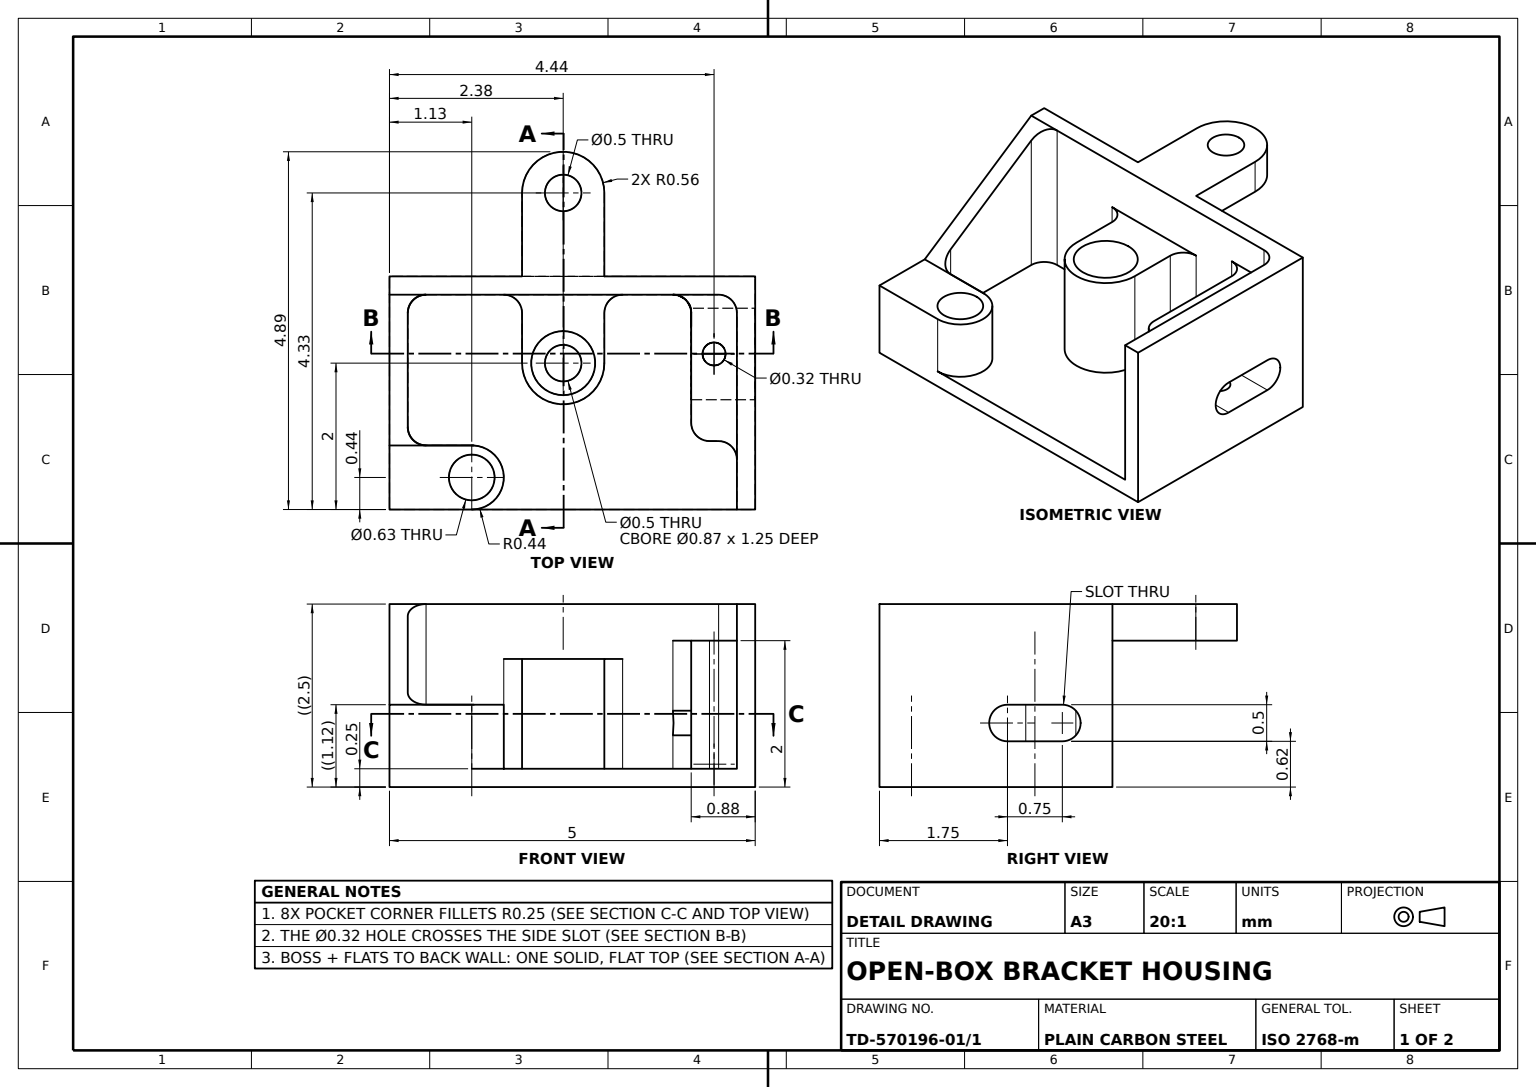
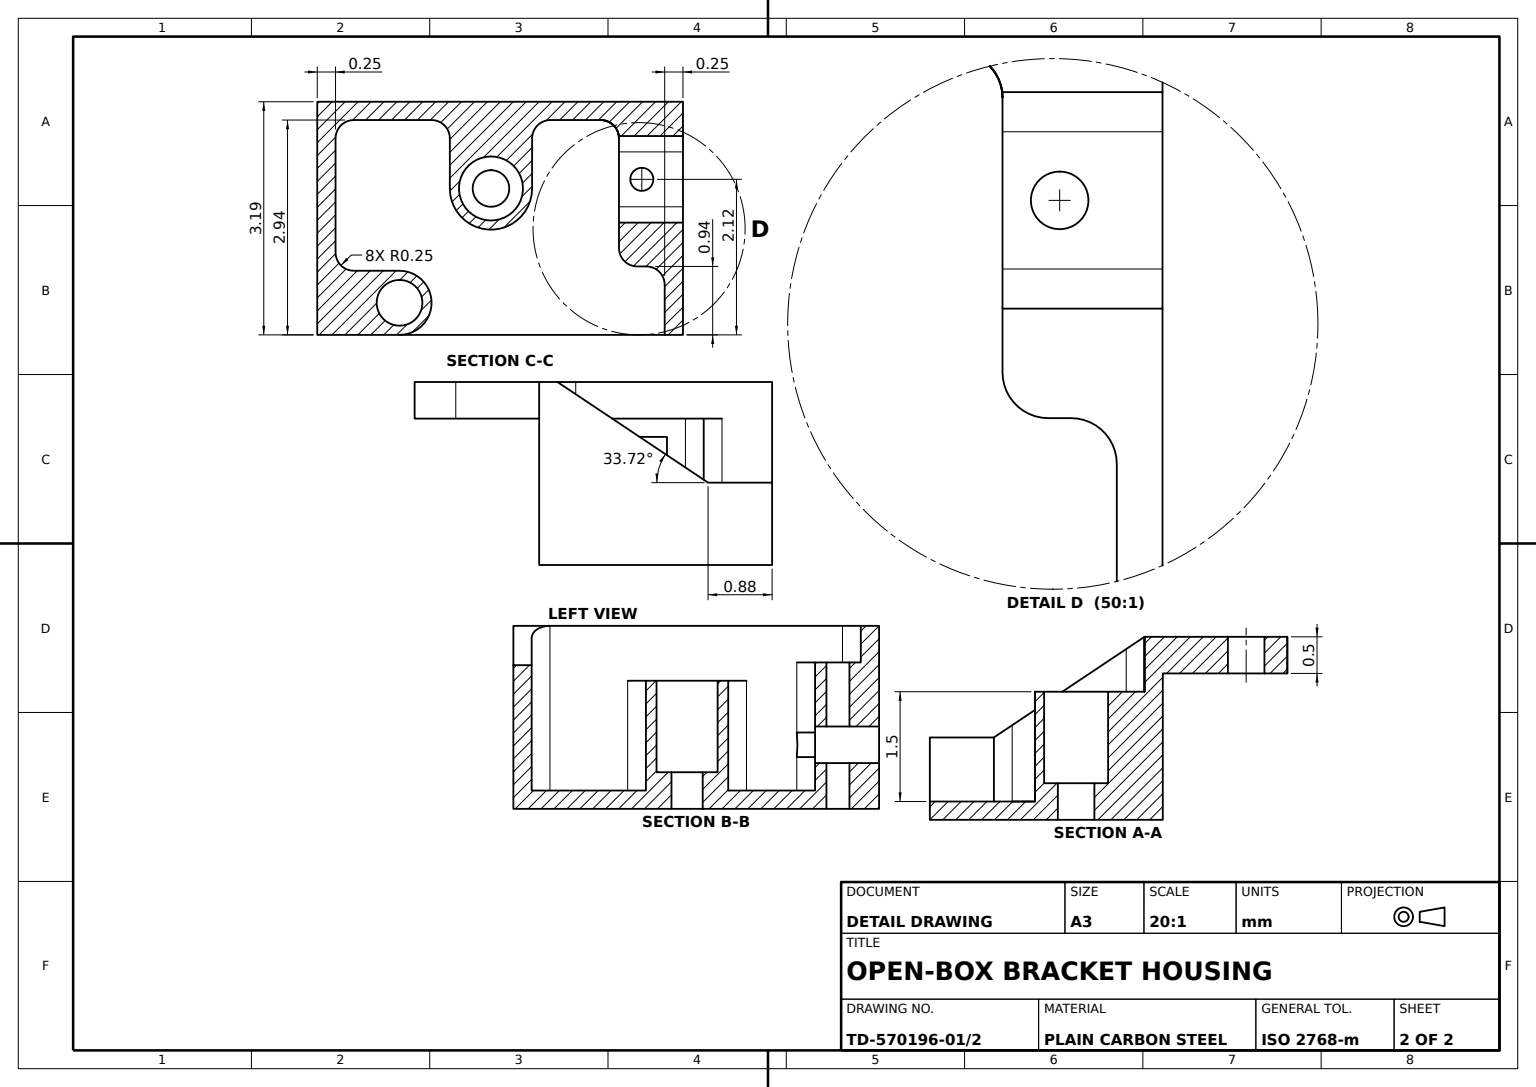
from build123d import *

# Parameters (mm, degrees)
BASE_PLATE_DEPTH              = 0.25
PERIMETER_WALLS_DEPTH         = 2.25
CORNER_BOSS_DEPTH             = 1.125
WALL_POCKET_CUT_DEPTH         = 2.125
CENTRAL_BOSS_DEPTH            = 1.5
MOUNTING_TAB_DEPTH            = 1.75
SIDE_WALL_SLOT_DEPTH          = 1.75
WALL_LIP_DEPTH                = 0.5
PROFILE_TRIM_SKETCH_R         = 0.25
PROFILE_TRIM_SKETCH_R_2       = 0.1575
PROFILE_TRIM_SKETCH_R_3       = 0.2205
PROFILE_TRIM_CUT_DEPTH        = 3.5
TAB_EDGE_FILLET_R0_25_R       = 0.25
TAB_WALL_FILLET_1_R0_25_R     = 0.25
TAB_WALL_FILLET_2_R0_25_R     = 0.25
CENTRAL_BOSS_FILLET_1_R0_25_R = 0.25
CENTRAL_BOSS_FILLET_2_R0_25_R = 0.25
WALL_FILLET_1_R0_25_R         = 0.25
CORNER_BOSS_FILLET_R0_25_R    = 0.25
WALL_FILLET_2_R0_25_R         = 0.25
BOSS_HOLE_SKETCH_0_875_R      = 0.4375
BOSS_HOLE_0_875_DEPTH         = 1.25
HOLE_SKETCH_0_625_R           = 0.3125
HOLE_0_625_DEPTH              = 1.25


with BuildPart() as part:
    # Base Plate Sketch → Base Plate (new body)
    with BuildSketch(Plane(origin=(0, 0, 0), x_dir=(1, 0, 0), z_dir=(0, 1, 0))):
        Polygon((0, 0), (2.5, 0), (2.5, 3.185), (-2.5, 3.185), (-2.5, 0), align=None)
    extrude(amount=BASE_PLATE_DEPTH)

    # Perimeter Walls Sketch → Perimeter Walls (add)
    with BuildSketch(Plane(origin=(0, 0.25, 0), x_dir=(1, 0, 0), z_dir=(0, 1, 0))):
        Polygon((-2.5, 0), (-2.5, 3.185), (2.5, 3.185), (2.5, 0), (2.25, 0), (2.25, 2.935), (-2.25, 2.935), (-2.25, 0), align=None)
    extrude(amount=PERIMETER_WALLS_DEPTH)

    # Corner Boss Sketch → Corner Boss (add)
    with BuildSketch(Plane(origin=(0, 0.25, 0), x_dir=(1, 0, 0), z_dir=(0, 1, 0))):
        with BuildLine():
            Line((-2.5, 0), (-2.5, 0.438))
            Line((-2.5, 0.438), (-2.5, 0.876))
            Line((-2.5, 0.876), (-1.375, 0.876))
            ThreePointArc((-1.375, 0.876), (-0.937, 0.438), (-1.375, 0))
            Line((-1.375, 0), (-2.5, 0))
        make_face()
    extrude(amount=CORNER_BOSS_DEPTH)

    # Wall Pocket Sketch → Wall Pocket Cut (cut)
    with BuildSketch(Plane.ZY.offset(2.5)):
        Polygon((0, 2.5), (-2.935, 2.5), (-0.875, 1.125), (0, 1.125), align=None)
    extrude(amount=-WALL_POCKET_CUT_DEPTH, mode=Mode.SUBTRACT)

    # Central Boss Sketch → Central Boss (add)
    with BuildSketch(Plane(origin=(0, 0.25, 0), x_dir=(1, 0, 0), z_dir=(0, 1, 0))):
        with BuildLine():
            ThreePointArc((-0.6875, 2), (-0.125, 1.4375), (0.4375, 2))
            Line((0.4375, 2), (0.4375, 2.935))
            Line((0.4375, 2.935), (0.4375, 3.185))
            Line((0.4375, 3.185), (-0.6875, 3.185))
            Line((-0.6875, 3.185), (-0.6875, 2))
        make_face()
    extrude(amount=CENTRAL_BOSS_DEPTH)

    # Mounting Tab Sketch → Mounting Tab (add)
    with BuildSketch(Plane(origin=(0, 0.25, 0), x_dir=(1, 0, 0), z_dir=(0, 1, 0))):
        Polygon((2.5, 3.185), (2.5, 0.935), (1.625, 0.935), (1.625, 2.935), (1.625, 3.185), align=None)
    extrude(amount=MOUNTING_TAB_DEPTH)

    # Side Slot Sketch → Side Wall Slot (cut)
    with BuildSketch(Plane(origin=(2.5, 0, 0), x_dir=(0, 0, -1), z_dir=(1, 0, 0))):
        with BuildLine():
            Line((1.75, 1.125), (2.5, 1.125))
            ThreePointArc((2.5, 1.125), (2.75, 0.875), (2.5, 0.625))
            Line((2.5, 0.625), (1.75, 0.625))
            ThreePointArc((1.75, 0.625), (1.5, 0.875), (1.75, 1.125))
        make_face()
    extrude(amount=-SIDE_WALL_SLOT_DEPTH, mode=Mode.SUBTRACT)

    # Wall Lip Sketch → Wall Lip (add)
    with BuildSketch(Plane(origin=(0, 2.5, 0), x_dir=(1, 0, 0), z_dir=(0, 1, 0))):
        with BuildLine():
            Line((-0.6875, 2.935), (0.4375, 2.935))
            Line((0.4375, 2.935), (0.4375, 4.325))
            ThreePointArc((0.4375, 4.325), (-0.125, 4.8875), (-0.6875, 4.325))
            Line((-0.6875, 4.325), (-0.6875, 2.935))
        make_face()
    extrude(amount=-WALL_LIP_DEPTH)

    # Profile Trim Sketch → Profile Trim Cut (cut)
    with BuildSketch(Plane(origin=(0, 2.5, 0), x_dir=(1, 0, 0), z_dir=(0, 1, 0))):
        with Locations(Location((-0.125, 4.325, 0), (0, 0, 270))):
            Circle(PROFILE_TRIM_SKETCH_R)
        with Locations(Location((1.9375, 2.125, 0), (0, 0, 270))):
            Circle(PROFILE_TRIM_SKETCH_R_2)
        with Locations(Location((-1.375, 0.438, 0), (0, 0, 270))):
            Circle(PROFILE_TRIM_SKETCH_R_3)
        with Locations(Location((-0.125, 2, 0), (0, 0, 270))):
            Circle(PROFILE_TRIM_SKETCH_R)
    extrude(amount=-PROFILE_TRIM_CUT_DEPTH, mode=Mode.SUBTRACT)

    # Tab Edge Fillet R0.25
    tab_edge_fillet_r0_25_edges = [part.edges().sort_by_distance(p)[0] for p in [
        (1.625, 1.125, -0.935),
    ]]
    fillet(tab_edge_fillet_r0_25_edges, radius=TAB_EDGE_FILLET_R0_25_R)

    # Tab-Wall Fillet 1 R0.25
    tab_wall_fillet_1_r0_25_edges = [part.edges().sort_by_distance(p)[0] for p in [
        (2.25, 1.125, -0.935),
    ]]
    fillet(tab_wall_fillet_1_r0_25_edges, radius=TAB_WALL_FILLET_1_R0_25_R)

    # Tab-Wall Fillet 2 R0.25
    tab_wall_fillet_2_r0_25_edges = [part.edges().sort_by_distance(p)[0] for p in [
        (1.625, 1.125, -2.935),
    ]]
    fillet(tab_wall_fillet_2_r0_25_edges, radius=TAB_WALL_FILLET_2_R0_25_R)

    # Central Boss Fillet 1 R0.25
    central_boss_fillet_1_r0_25_edges = [part.edges().sort_by_distance(p)[0] for p in [
        (0.4375, 1, -2.935),
    ]]
    fillet(central_boss_fillet_1_r0_25_edges, radius=CENTRAL_BOSS_FILLET_1_R0_25_R)

    # Central Boss Fillet 2 R0.25
    central_boss_fillet_2_r0_25_edges = [part.edges().sort_by_distance(p)[0] for p in [
        (-0.6875, 1, -2.935),
    ]]
    fillet(central_boss_fillet_2_r0_25_edges, radius=CENTRAL_BOSS_FILLET_2_R0_25_R)

    # Wall Fillet 1 R0.25
    wall_fillet_1_r0_25_edges = [part.edges().sort_by_distance(p)[0] for p in [
        (-2.25, 1.375, -2.935),
    ]]
    fillet(wall_fillet_1_r0_25_edges, radius=WALL_FILLET_1_R0_25_R)

    # Corner Boss Fillet R0.25
    corner_boss_fillet_r0_25_edges = [part.edges().sort_by_distance(p)[0] for p in [
        (-2.25, 0.687833738, -0.876),
    ]]
    fillet(corner_boss_fillet_r0_25_edges, radius=CORNER_BOSS_FILLET_R0_25_R)

    # Wall Fillet 2 R0.25
    wall_fillet_2_r0_25_edges = [part.edges().sort_by_distance(p)[0] for p in [
        (2.25, 2.25, -2.935),
    ]]
    fillet(wall_fillet_2_r0_25_edges, radius=WALL_FILLET_2_R0_25_R)

    # Boss Hole Sketch Ø0.875 → Boss Hole Ø0.875 (cut)
    with BuildSketch(Plane(origin=(0, 1.75, 0), x_dir=(1, 0, 0), z_dir=(0, 1, 0))):
        with Locations(Location((-0.125, 2, 0), (0, 0, 270))):
            Circle(BOSS_HOLE_SKETCH_0_875_R)
    extrude(amount=-BOSS_HOLE_0_875_DEPTH, mode=Mode.SUBTRACT)

    # Hole Sketch Ø0.625 → Hole Ø0.625 (cut)
    with BuildSketch(Plane(origin=(0, 1.125, 0), x_dir=(1, 0, 0), z_dir=(0, 1, 0))):
        with Locations(Location((-1.375, 0.438, 0), (0, 0, 270))):
            Circle(HOLE_SKETCH_0_625_R)
    extrude(amount=-HOLE_0_625_DEPTH, mode=Mode.SUBTRACT)


solid = part.part
